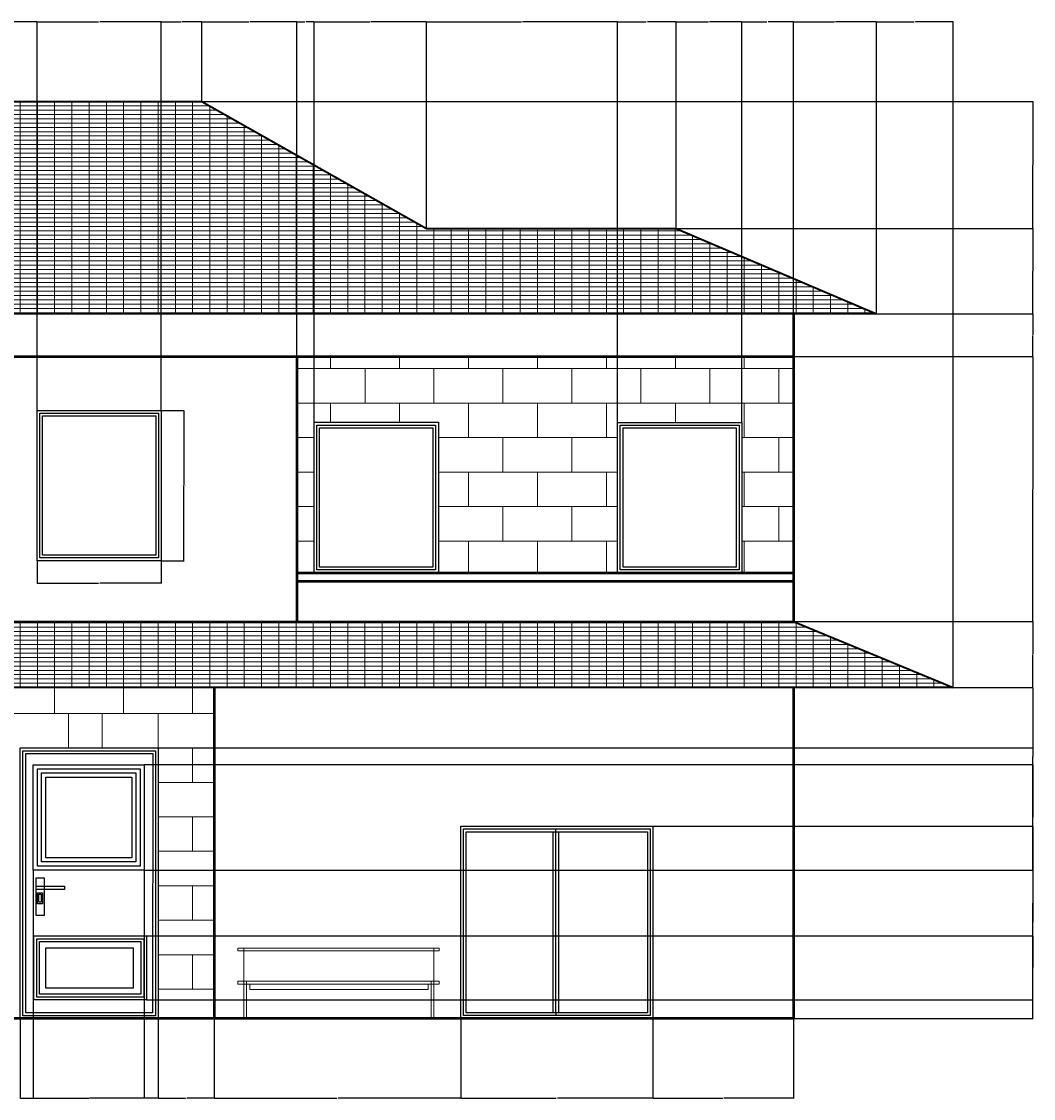
# Model space of a CAD drawing. Units: inches. Extents: x 357 to 1610, y 271 to 1052.
# Tile 2 of 2: x 876 to 1610, y 271 to 1052. Entities that reach past the tile are written whole.
import ezdxf

# ---------------------------------------------------------------- set-up
doc = ezdxf.new("R2010")
doc.units = ezdxf.units.IN
doc.header["$MEASUREMENT"] = 0
for name, color, linetype, lineweight in [('A-ANNO-DIMS', 2, 'Continuous', 18), ('A-DOOR', 40, 'Continuous', 25), ('A-FURN', 40, 'Continuous', 18), ('A-GLAZ', 4, 'Continuous', 25), ('A-ROOF', 7, 'Continuous', 35), ('A-ROOF-PATT', 8, 'Continuous', 13), ('A-WALL', 7, 'Continuous', 50), ('A-WALL-PATT', 8, 'Continuous', 18)]:
    doc.layers.add(name, color=color, linetype=linetype, lineweight=lineweight)
doc.styles.get("Standard").update_dxf_attribs({"font": 'arial.ttf'})
doc.dimstyles.get("Standard").update_dxf_attribs({"dimtxt": 0.18, "dimasz": 0.18, "dimexe": 0.18, "dimexo": 0.0625, "dimgap": 0.09, "dimtad": 0, "dimtih": 1, "dimtoh": 1, "dimdec": 4, "dimzin": 0, "dimdsep": 46, "dimtxsty": 'Standard', "dimcen": 0.09, "dimadec": 0, "dimazin": 0, "dimtfac": 1, "dimtdec": 4, "dimtofl": 0, "dimtmove": 0, "dimatfit": 3, "dimfxl": 1, "dimtolj": 1, "dimtzin": 0, "dimarcsym": 0})

# ---------------------------------------------------------------- blocks, each defined once
blk = doc.blocks.new('WIN-900x1090')
for points in [[(0, 108.96), (90.12, 108.96), (90.12, 0), (0, 0)], [(2, 106.96), (88.12, 106.96), (88.12, 2), (2, 2)], [(4, 104.96), (86.12, 104.96), (86.12, 4), (4, 4)]]:
    blk.add_lwpolyline(points, close=True)
blk = doc.blocks.new('*D2')
at = {"layer": 'A-ANNO-DIMS', "color": 0, "lineweight": -2, "transparency": 16777216}
for p, q in [((977.41, 769.73), (993.87, 769.73)), ((993.69, 769.55), (993.69, 715.44)), ((993.69, 660.95), (993.69, 715.07)), ((977.41, 660.77), (993.87, 660.77))]:
    blk.add_line(p, q, dxfattribs=at)
at = {"layer": 'A-ANNO-DIMS', "color": 0, "transparency": 16777216}
for points in [[(993.66, 769.55), (993.72, 769.55), (993.69, 769.73)], [(993.66, 660.95), (993.72, 660.95), (993.69, 660.77)]]:
    blk.add_solid(points, dxfattribs=at)
at = {"layer": 'Defpoints', "color": 0, "transparency": 16777216}
for p in [(977.34, 769.73), (993.69, 769.73), (977.34, 660.77)]:
    blk.add_point(p, dxfattribs=at)
at = {"layer": 'A-ANNO-DIMS', "color": 0, "transparency": 16777216, "insert": (993.69, 715.25), "char_height": 0.18, "attachment_point": 5}
blk.add_mtext('\\A1;WINDOW 900X1090 109 TYP.', dxfattribs=at)
blk = doc.blocks.new('*D3')
at = {"layer": 'A-ANNO-DIMS', "color": 0, "lineweight": -2, "transparency": 16777216}
for p, q in [((887.22, 660.71), (887.22, 644.25)), ((977.34, 660.71), (977.34, 644.25)), ((887.4, 644.43), (931.75, 644.43)), ((977.16, 644.43), (932.81, 644.43))]:
    blk.add_line(p, q, dxfattribs=at)
at = {"layer": 'A-ANNO-DIMS', "color": 0, "transparency": 16777216}
for points in [[(887.4, 644.46), (887.4, 644.4), (887.22, 644.43)], [(977.16, 644.46), (977.16, 644.4), (977.34, 644.43)]]:
    blk.add_solid(points, dxfattribs=at)
at = {"layer": 'Defpoints', "color": 0, "transparency": 16777216}
for p in [(887.22, 660.77), (977.34, 660.77), (977.34, 644.43)]:
    blk.add_point(p, dxfattribs=at)
at = {"layer": 'A-ANNO-DIMS', "color": 0, "transparency": 16777216, "insert": (932.28, 644.43), "char_height": 0.18, "attachment_point": 5}
blk.add_mtext('\\A1;90 TYP.', dxfattribs=at)
blk = doc.blocks.new('*D10')
at = {"layer": 'A-ANNO-DIMS', "color": 0, "lineweight": -2, "transparency": 16777216}
for p, q in [((835.67, 808.83), (835.67, 1051.75)), ((835.85, 1051.57), (861.05, 1051.57)), ((887.04, 1051.57), (861.84, 1051.57)), ((887.22, 769.8), (887.22, 1051.75))]:
    blk.add_line(p, q, dxfattribs=at)
at = {"layer": 'A-ANNO-DIMS', "color": 0, "transparency": 16777216}
for points in [[(835.85, 1051.6), (835.85, 1051.54), (835.67, 1051.57)], [(887.04, 1051.6), (887.04, 1051.54), (887.22, 1051.57)]]:
    blk.add_solid(points, dxfattribs=at)
at = {"layer": 'Defpoints', "color": 0, "transparency": 16777216}
for p in [(887.22, 1051.57), (835.67, 808.77), (887.22, 769.73)]:
    blk.add_point(p, dxfattribs=at)
at = {"layer": 'A-ANNO-DIMS', "color": 0, "transparency": 16777216, "insert": (861.44, 1051.57), "char_height": 0.18, "attachment_point": 5}
blk.add_mtext('\\A1;51.55', dxfattribs=at)
blk = doc.blocks.new('*D11')
at = {"layer": 'A-ANNO-DIMS', "color": 0, "lineweight": -2, "transparency": 16777216}
for p, q in [((887.22, 769.8), (887.22, 1051.75)), ((887.4, 1051.57), (931.89, 1051.57)), ((977.16, 1051.57), (932.67, 1051.57)), ((977.34, 769.8), (977.34, 1051.75))]:
    blk.add_line(p, q, dxfattribs=at)
at = {"layer": 'A-ANNO-DIMS', "color": 0, "transparency": 16777216}
for points in [[(887.4, 1051.6), (887.4, 1051.54), (887.22, 1051.57)], [(977.16, 1051.6), (977.16, 1051.54), (977.34, 1051.57)]]:
    blk.add_solid(points, dxfattribs=at)
at = {"layer": 'Defpoints', "color": 0, "transparency": 16777216}
for p in [(977.34, 1051.57), (887.22, 769.73), (977.34, 769.73)]:
    blk.add_point(p, dxfattribs=at)
at = {"layer": 'A-ANNO-DIMS', "color": 0, "transparency": 16777216, "insert": (932.28, 1051.57), "char_height": 0.18, "attachment_point": 5}
blk.add_mtext('\\A1;90.12', dxfattribs=at)
blk = doc.blocks.new('*D12')
at = {"layer": 'A-ANNO-DIMS', "color": 0, "lineweight": -2, "transparency": 16777216}
for p, q in [((977.34, 769.8), (977.34, 1051.75)), ((977.52, 1051.57), (991.72, 1051.57)), ((1006.56, 1051.57), (992.37, 1051.57)), ((1006.74, 993.83), (1006.74, 1051.75))]:
    blk.add_line(p, q, dxfattribs=at)
at = {"layer": 'A-ANNO-DIMS', "color": 0, "transparency": 16777216}
for points in [[(977.52, 1051.6), (977.52, 1051.54), (977.34, 1051.57)], [(1006.56, 1051.6), (1006.56, 1051.54), (1006.74, 1051.57)]]:
    blk.add_solid(points, dxfattribs=at)
at = {"layer": 'Defpoints', "color": 0, "transparency": 16777216}
for p in [(1006.74, 1051.57), (1006.74, 993.77), (977.34, 769.73)]:
    blk.add_point(p, dxfattribs=at)
at = {"layer": 'A-ANNO-DIMS', "color": 0, "transparency": 16777216, "insert": (992.04, 1051.57), "char_height": 0.18, "attachment_point": 5}
blk.add_mtext('\\A1;29.4', dxfattribs=at)
blk = doc.blocks.new('*D13')
at = {"layer": 'A-ANNO-DIMS', "color": 0, "lineweight": -2, "transparency": 16777216}
for p, q in [((1006.74, 993.83), (1006.74, 1051.75)), ((1006.92, 1051.57), (1040.81, 1051.57)), ((1075.49, 1051.57), (1041.6, 1051.57)), ((1075.67, 808.83), (1075.67, 1051.75))]:
    blk.add_line(p, q, dxfattribs=at)
at = {"layer": 'A-ANNO-DIMS', "color": 0, "transparency": 16777216}
for points in [[(1006.92, 1051.6), (1006.92, 1051.54), (1006.74, 1051.57)], [(1075.49, 1051.6), (1075.49, 1051.54), (1075.67, 1051.57)]]:
    blk.add_solid(points, dxfattribs=at)
at = {"layer": 'Defpoints', "color": 0, "transparency": 16777216}
for p in [(1075.67, 1051.57), (1006.74, 993.77), (1075.67, 808.77)]:
    blk.add_point(p, dxfattribs=at)
at = {"layer": 'A-ANNO-DIMS', "color": 0, "transparency": 16777216, "insert": (1041.21, 1051.57), "char_height": 0.18, "attachment_point": 5}
blk.add_mtext('\\A1;68.93', dxfattribs=at)
blk = doc.blocks.new('*D14')
at = {"layer": 'A-ANNO-DIMS', "color": 0, "lineweight": -2, "transparency": 16777216}
for p, q in [((1075.67, 808.83), (1075.67, 1051.75)), ((1075.85, 1051.57), (1081.44, 1051.57)), ((1087.93, 1051.57), (1082.35, 1051.57)), ((1088.11, 761.21), (1088.11, 1051.75))]:
    blk.add_line(p, q, dxfattribs=at)
at = {"layer": 'A-ANNO-DIMS', "color": 0, "transparency": 16777216}
for points in [[(1075.85, 1051.6), (1075.85, 1051.54), (1075.67, 1051.57)], [(1087.93, 1051.6), (1087.93, 1051.54), (1088.11, 1051.57)]]:
    blk.add_solid(points, dxfattribs=at)
at = {"layer": 'Defpoints', "color": 0, "transparency": 16777216}
for p in [(1088.11, 1051.57), (1075.67, 808.77), (1088.11, 761.15)]:
    blk.add_point(p, dxfattribs=at)
at = {"layer": 'A-ANNO-DIMS', "color": 0, "transparency": 16777216, "insert": (1081.89, 1051.57), "char_height": 0.18, "attachment_point": 5}
blk.add_mtext('\\A1;12.443', dxfattribs=at)
blk = doc.blocks.new('*D15')
at = {"layer": 'A-ANNO-DIMS', "color": 0, "lineweight": -2, "transparency": 16777216}
for p, q in [((1088.11, 761.21), (1088.11, 1051.75)), ((1088.29, 1051.57), (1128.49, 1051.57)), ((1169.34, 1051.57), (1129.14, 1051.57)), ((1169.52, 901.81), (1169.52, 1051.75))]:
    blk.add_line(p, q, dxfattribs=at)
at = {"layer": 'A-ANNO-DIMS', "color": 0, "transparency": 16777216}
for points in [[(1088.29, 1051.6), (1088.29, 1051.54), (1088.11, 1051.57)], [(1169.34, 1051.6), (1169.34, 1051.54), (1169.52, 1051.57)]]:
    blk.add_solid(points, dxfattribs=at)
at = {"layer": 'Defpoints', "color": 0, "transparency": 16777216}
for p in [(1169.52, 1051.57), (1169.52, 901.75), (1088.11, 761.15)]:
    blk.add_point(p, dxfattribs=at)
at = {"layer": 'A-ANNO-DIMS', "color": 0, "transparency": 16777216, "insert": (1128.82, 1051.57), "char_height": 0.18, "attachment_point": 5}
blk.add_mtext('\\A1;81.4', dxfattribs=at)
blk = doc.blocks.new('*D16')
at = {"layer": 'A-ANNO-DIMS', "color": 0, "lineweight": -2, "transparency": 16777216}
for p, q in [((1169.52, 901.81), (1169.52, 1051.75)), ((1169.7, 1051.57), (1238.43, 1051.57)), ((1307.93, 1051.57), (1239.2, 1051.57)), ((1308.11, 761.12), (1308.11, 1051.75))]:
    blk.add_line(p, q, dxfattribs=at)
at = {"layer": 'A-ANNO-DIMS', "color": 0, "transparency": 16777216}
for points in [[(1169.7, 1051.6), (1169.7, 1051.54), (1169.52, 1051.57)], [(1307.93, 1051.6), (1307.93, 1051.54), (1308.11, 1051.57)]]:
    blk.add_solid(points, dxfattribs=at)
at = {"layer": 'Defpoints', "color": 0, "transparency": 16777216}
for p in [(1308.11, 1051.57), (1169.52, 901.75), (1308.11, 761.06)]:
    blk.add_point(p, dxfattribs=at)
at = {"layer": 'A-ANNO-DIMS', "color": 0, "transparency": 16777216, "insert": (1238.81, 1051.57), "char_height": 0.18, "attachment_point": 5}
blk.add_mtext('\\A1;138.6', dxfattribs=at)
blk = doc.blocks.new('*D17')
at = {"layer": 'A-ANNO-DIMS', "color": 0, "lineweight": -2, "transparency": 16777216}
for p, q in [((1308.11, 761.12), (1308.11, 1051.75)), ((1308.29, 1051.57), (1328.95, 1051.57)), ((1350.4, 1051.57), (1329.74, 1051.57)), ((1350.58, 901.81), (1350.58, 1051.75))]:
    blk.add_line(p, q, dxfattribs=at)
at = {"layer": 'A-ANNO-DIMS', "color": 0, "transparency": 16777216}
for points in [[(1308.29, 1051.6), (1308.29, 1051.54), (1308.11, 1051.57)], [(1350.4, 1051.6), (1350.4, 1051.54), (1350.58, 1051.57)]]:
    blk.add_solid(points, dxfattribs=at)
at = {"layer": 'Defpoints', "color": 0, "transparency": 16777216}
for p in [(1350.58, 1051.57), (1350.58, 901.75), (1308.11, 761.06)]:
    blk.add_point(p, dxfattribs=at)
at = {"layer": 'A-ANNO-DIMS', "color": 0, "transparency": 16777216, "insert": (1329.35, 1051.57), "char_height": 0.18, "attachment_point": 5}
blk.add_mtext('\\A1;42.48', dxfattribs=at)
blk = doc.blocks.new('*D18')
at = {"layer": 'A-ANNO-DIMS', "color": 0, "lineweight": -2, "transparency": 16777216}
for p, q in [((1350.58, 901.81), (1350.58, 1051.75)), ((1350.76, 1051.57), (1374.01, 1051.57)), ((1398.05, 1051.57), (1374.81, 1051.57)), ((1398.23, 761.12), (1398.23, 1051.75))]:
    blk.add_line(p, q, dxfattribs=at)
at = {"layer": 'A-ANNO-DIMS', "color": 0, "transparency": 16777216}
for points in [[(1350.76, 1051.6), (1350.76, 1051.54), (1350.58, 1051.57)], [(1398.05, 1051.6), (1398.05, 1051.54), (1398.23, 1051.57)]]:
    blk.add_solid(points, dxfattribs=at)
at = {"layer": 'Defpoints', "color": 0, "transparency": 16777216}
for p in [(1398.23, 1051.57), (1350.58, 901.75), (1398.23, 761.06)]:
    blk.add_point(p, dxfattribs=at)
at = {"layer": 'A-ANNO-DIMS', "color": 0, "transparency": 16777216, "insert": (1374.41, 1051.57), "char_height": 0.18, "attachment_point": 5}
blk.add_mtext('\\A1;47.65', dxfattribs=at)
blk = doc.blocks.new('*D19')
at = {"layer": 'A-ANNO-DIMS', "color": 0, "lineweight": -2, "transparency": 16777216}
for p, q in [((1398.23, 761.12), (1398.23, 1051.75)), ((1398.41, 1051.57), (1416.45, 1051.57)), ((1435.41, 1051.57), (1417.37, 1051.57)), ((1435.59, 839.95), (1435.59, 1051.75))]:
    blk.add_line(p, q, dxfattribs=at)
at = {"layer": 'A-ANNO-DIMS', "color": 0, "transparency": 16777216}
for points in [[(1398.41, 1051.6), (1398.41, 1051.54), (1398.23, 1051.57)], [(1435.41, 1051.6), (1435.41, 1051.54), (1435.59, 1051.57)]]:
    blk.add_solid(points, dxfattribs=at)
at = {"layer": 'Defpoints', "color": 0, "transparency": 16777216}
for p in [(1435.59, 1051.57), (1435.59, 839.89), (1398.23, 761.06)]:
    blk.add_point(p, dxfattribs=at)
at = {"layer": 'A-ANNO-DIMS', "color": 0, "transparency": 16777216, "insert": (1416.91, 1051.57), "char_height": 0.18, "attachment_point": 5}
blk.add_mtext('\\A1;37.356', dxfattribs=at)
blk = doc.blocks.new('*D20')
at = {"layer": 'A-ANNO-DIMS', "color": 0, "lineweight": -2, "transparency": 16777216}
for p, q in [((1435.59, 839.95), (1435.59, 1051.75)), ((1435.77, 1051.57), (1465.3, 1051.57)), ((1495.63, 1051.57), (1466.09, 1051.57)), ((1495.81, 839.95), (1495.81, 1051.75))]:
    blk.add_line(p, q, dxfattribs=at)
at = {"layer": 'A-ANNO-DIMS', "color": 0, "transparency": 16777216}
for points in [[(1435.77, 1051.6), (1435.77, 1051.54), (1435.59, 1051.57)], [(1495.63, 1051.6), (1495.63, 1051.54), (1495.81, 1051.57)]]:
    blk.add_solid(points, dxfattribs=at)
at = {"layer": 'Defpoints', "color": 0, "transparency": 16777216}
for p in [(1495.81, 1051.57), (1435.59, 839.89), (1495.81, 839.89)]:
    blk.add_point(p, dxfattribs=at)
at = {"layer": 'A-ANNO-DIMS', "color": 0, "transparency": 16777216, "insert": (1465.7, 1051.57), "char_height": 0.18, "attachment_point": 5}
blk.add_mtext('\\A1;60.22', dxfattribs=at)
blk = doc.blocks.new('*D21')
at = {"layer": 'A-ANNO-DIMS', "color": 0, "lineweight": -2, "transparency": 16777216}
for p, q in [((1495.81, 839.95), (1495.81, 1051.75)), ((1495.99, 1051.57), (1523.25, 1051.57)), ((1551.3, 1051.57), (1524.04, 1051.57)), ((1551.48, 568.83), (1551.48, 1051.75))]:
    blk.add_line(p, q, dxfattribs=at)
at = {"layer": 'A-ANNO-DIMS', "color": 0, "transparency": 16777216}
for points in [[(1495.99, 1051.6), (1495.99, 1051.54), (1495.81, 1051.57)], [(1551.3, 1051.6), (1551.3, 1051.54), (1551.48, 1051.57)]]:
    blk.add_solid(points, dxfattribs=at)
at = {"layer": 'Defpoints', "color": 0, "transparency": 16777216}
for p in [(1551.48, 1051.57), (1495.81, 839.89), (1551.48, 568.77)]:
    blk.add_point(p, dxfattribs=at)
at = {"layer": 'A-ANNO-DIMS', "color": 0, "transparency": 16777216, "insert": (1523.64, 1051.57), "char_height": 0.18, "attachment_point": 5}
blk.add_mtext('\\A1;55.67', dxfattribs=at)
blk = doc.blocks.new('*D27')
at = {"layer": 'A-ANNO-DIMS', "color": 0, "lineweight": -2, "transparency": 16777216}
for p, q in [((875, 328.7), (875, 270.79)), ((975, 328.7), (975, 270.79)), ((875.18, 270.97), (924.72, 270.97)), ((974.82, 270.97), (925.28, 270.97))]:
    blk.add_line(p, q, dxfattribs=at)
at = {"layer": 'A-ANNO-DIMS', "color": 0, "transparency": 16777216}
for points in [[(875.18, 271), (875.18, 270.94), (875, 270.97)], [(974.82, 271), (974.82, 270.94), (975, 270.97)]]:
    blk.add_solid(points, dxfattribs=at)
at = {"layer": 'Defpoints', "color": 0, "transparency": 16777216}
for p in [(875, 328.77), (975, 328.77), (975, 270.97)]:
    blk.add_point(p, dxfattribs=at)
at = {"layer": 'A-ANNO-DIMS', "color": 0, "transparency": 16777216, "insert": (925, 270.97), "char_height": 0.18, "attachment_point": 5}
blk.add_mtext('\\A1;100', dxfattribs=at)
blk = doc.blocks.new('*D28')
at = {"layer": 'A-ANNO-DIMS', "color": 0, "lineweight": -2, "transparency": 16777216}
for p, q in [((975, 328.7), (975, 270.79)), ((1015.67, 328.7), (1015.67, 270.79)), ((975.18, 270.97), (994.94, 270.97)), ((1015.49, 270.97), (995.73, 270.97))]:
    blk.add_line(p, q, dxfattribs=at)
at = {"layer": 'A-ANNO-DIMS', "color": 0, "transparency": 16777216}
for points in [[(975.18, 271), (975.18, 270.94), (975, 270.97)], [(1015.49, 271), (1015.49, 270.94), (1015.67, 270.97)]]:
    blk.add_solid(points, dxfattribs=at)
at = {"layer": 'Defpoints', "color": 0, "transparency": 16777216}
for p in [(975, 328.77), (1015.67, 328.77), (1015.67, 270.97)]:
    blk.add_point(p, dxfattribs=at)
at = {"layer": 'A-ANNO-DIMS', "color": 0, "transparency": 16777216, "insert": (995.33, 270.97), "char_height": 0.18, "attachment_point": 5}
blk.add_mtext('\\A1;40.67', dxfattribs=at)
blk = doc.blocks.new('*D29')
at = {"layer": 'A-ANNO-DIMS', "color": 0, "lineweight": -2, "transparency": 16777216}
for p, q in [((1015.67, 328.7), (1015.67, 270.79)), ((1194.43, 328.82), (1194.43, 270.79)), ((1015.85, 270.97), (1104.6, 270.97)), ((1194.25, 270.97), (1105.51, 270.97))]:
    blk.add_line(p, q, dxfattribs=at)
at = {"layer": 'A-ANNO-DIMS', "color": 0, "transparency": 16777216}
for points in [[(1015.85, 271), (1015.85, 270.94), (1015.67, 270.97)], [(1194.25, 271), (1194.25, 270.94), (1194.43, 270.97)]]:
    blk.add_solid(points, dxfattribs=at)
at = {"layer": 'Defpoints', "color": 0, "transparency": 16777216}
for p in [(1015.67, 328.77), (1194.43, 328.88), (1194.43, 270.97)]:
    blk.add_point(p, dxfattribs=at)
at = {"layer": 'A-ANNO-DIMS', "color": 0, "transparency": 16777216, "insert": (1105.05, 270.97), "char_height": 0.18, "attachment_point": 5}
blk.add_mtext('\\A1;178.76', dxfattribs=at)
blk = doc.blocks.new('*D30')
at = {"layer": 'A-ANNO-DIMS', "color": 0, "lineweight": -2, "transparency": 16777216}
for p, q in [((1194.43, 328.82), (1194.43, 270.79)), ((1333.76, 328.82), (1333.76, 270.79)), ((1194.61, 270.97), (1263.64, 270.97)), ((1333.58, 270.97), (1264.55, 270.97))]:
    blk.add_line(p, q, dxfattribs=at)
at = {"layer": 'A-ANNO-DIMS', "color": 0, "transparency": 16777216}
for points in [[(1194.61, 271), (1194.61, 270.94), (1194.43, 270.97)], [(1333.58, 271), (1333.58, 270.94), (1333.76, 270.97)]]:
    blk.add_solid(points, dxfattribs=at)
at = {"layer": 'Defpoints', "color": 0, "transparency": 16777216}
for p in [(1194.43, 328.88), (1333.76, 328.88), (1333.76, 270.97)]:
    blk.add_point(p, dxfattribs=at)
at = {"layer": 'A-ANNO-DIMS', "color": 0, "transparency": 16777216, "insert": (1264.1, 270.97), "char_height": 0.18, "attachment_point": 5}
blk.add_mtext('\\A1;139.33', dxfattribs=at)
blk = doc.blocks.new('*D31')
at = {"layer": 'A-ANNO-DIMS', "color": 0, "lineweight": -2, "transparency": 16777216}
for p, q in [((1333.76, 328.82), (1333.76, 270.79)), ((1435.67, 328.7), (1435.67, 270.79)), ((1333.94, 270.97), (1384.33, 270.97)), ((1435.49, 270.97), (1385.1, 270.97))]:
    blk.add_line(p, q, dxfattribs=at)
at = {"layer": 'A-ANNO-DIMS', "color": 0, "transparency": 16777216}
for points in [[(1333.94, 271), (1333.94, 270.94), (1333.76, 270.97)], [(1435.49, 271), (1435.49, 270.94), (1435.67, 270.97)]]:
    blk.add_solid(points, dxfattribs=at)
at = {"layer": 'Defpoints', "color": 0, "transparency": 16777216}
for p in [(1333.76, 328.88), (1435.67, 328.77), (1435.67, 270.97)]:
    blk.add_point(p, dxfattribs=at)
at = {"layer": 'A-ANNO-DIMS', "color": 0, "transparency": 16777216, "insert": (1384.71, 270.97), "char_height": 0.18, "attachment_point": 5}
blk.add_mtext('\\A1;101.9', dxfattribs=at)
blk = doc.blocks.new('*D40')
at = {"layer": 'A-ANNO-DIMS', "color": 0, "lineweight": -2, "transparency": 16777216}
for p, q in [((1194.5, 468.2), (1609.46, 468.2)), ((1609.28, 468.02), (1609.28, 398.67)), ((1609.28, 328.95), (1609.28, 398.3)), ((1435.73, 328.77), (1609.46, 328.77))]:
    blk.add_line(p, q, dxfattribs=at)
at = {"layer": 'A-ANNO-DIMS', "color": 0, "transparency": 16777216}
for points in [[(1609.25, 468.02), (1609.31, 468.02), (1609.28, 468.2)], [(1609.25, 328.95), (1609.31, 328.95), (1609.28, 328.77)]]:
    blk.add_solid(points, dxfattribs=at)
at = {"layer": 'Defpoints', "color": 0, "transparency": 16777216}
for p in [(1194.43, 468.2), (1609.28, 468.2), (1435.67, 328.77)]:
    blk.add_point(p, dxfattribs=at)
at = {"layer": 'A-ANNO-DIMS', "color": 0, "transparency": 16777216, "insert": (1609.28, 398.49), "char_height": 0.18, "attachment_point": 5}
blk.add_mtext('\\A1;139.44', dxfattribs=at)
blk = doc.blocks.new('*D41')
at = {"layer": 'A-ANNO-DIMS', "color": 0, "lineweight": -2, "transparency": 16777216}
for p, q in [((1551.54, 568.77), (1609.46, 568.77)), ((1609.28, 568.59), (1609.28, 518.67)), ((1609.28, 468.38), (1609.28, 518.3)), ((1194.5, 468.2), (1609.46, 468.2))]:
    blk.add_line(p, q, dxfattribs=at)
at = {"layer": 'A-ANNO-DIMS', "color": 0, "transparency": 16777216}
for points in [[(1609.25, 568.59), (1609.31, 568.59), (1609.28, 568.77)], [(1609.25, 468.38), (1609.31, 468.38), (1609.28, 468.2)]]:
    blk.add_solid(points, dxfattribs=at)
at = {"layer": 'Defpoints', "color": 0, "transparency": 16777216}
for p in [(1551.48, 568.77), (1609.28, 568.77), (1194.43, 468.2)]:
    blk.add_point(p, dxfattribs=at)
at = {"layer": 'A-ANNO-DIMS', "color": 0, "transparency": 16777216, "insert": (1609.28, 518.49), "char_height": 0.18, "attachment_point": 5}
blk.add_mtext('\\A1;100.56', dxfattribs=at)
blk = doc.blocks.new('*D42')
at = {"layer": 'A-ANNO-DIMS', "color": 0, "lineweight": -2, "transparency": 16777216}
for p, q in [((1435.73, 616.77), (1609.46, 616.77)), ((1609.28, 616.59), (1609.28, 592.95)), ((1609.28, 568.95), (1609.28, 592.59)), ((1551.54, 568.77), (1609.46, 568.77))]:
    blk.add_line(p, q, dxfattribs=at)
at = {"layer": 'A-ANNO-DIMS', "color": 0, "transparency": 16777216}
for points in [[(1609.25, 616.59), (1609.31, 616.59), (1609.28, 616.77)], [(1609.25, 568.95), (1609.31, 568.95), (1609.28, 568.77)]]:
    blk.add_solid(points, dxfattribs=at)
at = {"layer": 'Defpoints', "color": 0, "transparency": 16777216}
for p in [(1435.67, 616.77), (1609.28, 616.77), (1551.48, 568.77)]:
    blk.add_point(p, dxfattribs=at)
at = {"layer": 'A-ANNO-DIMS', "color": 0, "transparency": 16777216, "insert": (1609.28, 592.77), "char_height": 0.18, "attachment_point": 5}
blk.add_mtext('\\A1;48', dxfattribs=at)
blk = doc.blocks.new('*D43')
at = {"layer": 'A-ANNO-DIMS', "color": 0, "lineweight": -2, "transparency": 16777216}
for p, q in [((1075.73, 808.77), (1609.46, 808.77)), ((1609.28, 808.59), (1609.28, 712.95)), ((1609.28, 616.95), (1609.28, 712.59)), ((1435.73, 616.77), (1609.46, 616.77))]:
    blk.add_line(p, q, dxfattribs=at)
at = {"layer": 'A-ANNO-DIMS', "color": 0, "transparency": 16777216}
for points in [[(1609.25, 808.59), (1609.31, 808.59), (1609.28, 808.77)], [(1609.25, 616.95), (1609.31, 616.95), (1609.28, 616.77)]]:
    blk.add_solid(points, dxfattribs=at)
at = {"layer": 'Defpoints', "color": 0, "transparency": 16777216}
for p in [(1075.67, 808.77), (1609.28, 808.77), (1435.67, 616.77)]:
    blk.add_point(p, dxfattribs=at)
at = {"layer": 'A-ANNO-DIMS', "color": 0, "transparency": 16777216, "insert": (1609.28, 712.77), "char_height": 0.18, "attachment_point": 5}
blk.add_mtext('\\A1;192', dxfattribs=at)
blk = doc.blocks.new('*D44')
at = {"layer": 'A-ANNO-DIMS', "color": 0, "lineweight": -2, "transparency": 16777216}
for p, q in [((1495.87, 839.89), (1609.46, 839.89)), ((1609.28, 839.71), (1609.28, 824.51)), ((1609.28, 808.95), (1609.28, 824.15)), ((1075.73, 808.77), (1609.46, 808.77))]:
    blk.add_line(p, q, dxfattribs=at)
at = {"layer": 'A-ANNO-DIMS', "color": 0, "transparency": 16777216}
for points in [[(1609.25, 839.71), (1609.31, 839.71), (1609.28, 839.89)], [(1609.25, 808.95), (1609.31, 808.95), (1609.28, 808.77)]]:
    blk.add_solid(points, dxfattribs=at)
at = {"layer": 'Defpoints', "color": 0, "transparency": 16777216}
for p in [(1495.81, 839.89), (1609.28, 839.89), (1075.67, 808.77)]:
    blk.add_point(p, dxfattribs=at)
at = {"layer": 'A-ANNO-DIMS', "color": 0, "transparency": 16777216, "insert": (1609.28, 824.33), "char_height": 0.18, "attachment_point": 5}
blk.add_mtext('\\A1;31.12', dxfattribs=at)
blk = doc.blocks.new('*D45')
at = {"layer": 'A-ANNO-DIMS', "color": 0, "lineweight": -2, "transparency": 16777216}
for p, q in [((1350.65, 901.75), (1609.46, 901.75)), ((1609.28, 901.57), (1609.28, 871)), ((1609.28, 840.07), (1609.28, 870.64)), ((1495.87, 839.89), (1609.46, 839.89))]:
    blk.add_line(p, q, dxfattribs=at)
at = {"layer": 'A-ANNO-DIMS', "color": 0, "transparency": 16777216}
for points in [[(1609.25, 901.57), (1609.31, 901.57), (1609.28, 901.75)], [(1609.25, 840.07), (1609.31, 840.07), (1609.28, 839.89)]]:
    blk.add_solid(points, dxfattribs=at)
at = {"layer": 'Defpoints', "color": 0, "transparency": 16777216}
for p in [(1350.58, 901.75), (1609.28, 901.75), (1495.81, 839.89)]:
    blk.add_point(p, dxfattribs=at)
at = {"layer": 'A-ANNO-DIMS', "color": 0, "transparency": 16777216, "insert": (1609.28, 870.82), "char_height": 0.18, "attachment_point": 5}
blk.add_mtext('\\A1;61.86', dxfattribs=at)
blk = doc.blocks.new('*D46')
at = {"layer": 'A-ANNO-DIMS', "color": 0, "lineweight": -2, "transparency": 16777216}
for p, q in [((1006.8, 993.77), (1609.46, 993.77)), ((1609.28, 993.59), (1609.28, 947.94)), ((1609.28, 901.93), (1609.28, 947.58)), ((1350.65, 901.75), (1609.46, 901.75))]:
    blk.add_line(p, q, dxfattribs=at)
at = {"layer": 'A-ANNO-DIMS', "color": 0, "transparency": 16777216}
for points in [[(1609.25, 993.59), (1609.31, 993.59), (1609.28, 993.77)], [(1609.25, 901.93), (1609.31, 901.93), (1609.28, 901.75)]]:
    blk.add_solid(points, dxfattribs=at)
at = {"layer": 'Defpoints', "color": 0, "transparency": 16777216}
for p in [(1006.74, 993.77), (1609.28, 993.77), (1350.58, 901.75)]:
    blk.add_point(p, dxfattribs=at)
at = {"layer": 'A-ANNO-DIMS', "color": 0, "transparency": 16777216, "insert": (1609.28, 947.76), "char_height": 0.18, "attachment_point": 5}
blk.add_mtext('\\A1;92.02', dxfattribs=at)
blk = doc.blocks.new('*D47')
at = {"layer": 'A-ANNO-DIMS', "color": 0, "lineweight": -2, "transparency": 16777216}
for p, q in [((966.64, 388.65), (1609.46, 388.65)), ((1609.28, 388.47), (1609.28, 365.69)), ((1609.28, 342.54), (1609.28, 365.32)), ((966.64, 342.36), (1609.46, 342.36))]:
    blk.add_line(p, q, dxfattribs=at)
at = {"layer": 'A-ANNO-DIMS', "color": 0, "transparency": 16777216}
for points in [[(1609.25, 388.47), (1609.31, 388.47), (1609.28, 388.65)], [(1609.25, 342.54), (1609.31, 342.54), (1609.28, 342.36)]]:
    blk.add_solid(points, dxfattribs=at)
at = {"layer": 'Defpoints', "color": 0, "transparency": 16777216}
for p in [(966.57, 388.65), (1609.28, 388.65), (966.57, 342.36)]:
    blk.add_point(p, dxfattribs=at)
at = {"layer": 'A-ANNO-DIMS', "color": 0, "transparency": 16777216, "insert": (1609.28, 365.51), "char_height": 0.18, "attachment_point": 5}
blk.add_mtext('\\A1;46.3', dxfattribs=at)
blk = doc.blocks.new('*D48')
at = {"layer": 'A-ANNO-DIMS', "color": 0, "lineweight": -2, "transparency": 16777216}
for p, q in [((965.04, 436.35), (1609.46, 436.35)), ((1609.28, 436.17), (1609.28, 412.68)), ((1609.28, 388.83), (1609.28, 412.32)), ((966.64, 388.65), (1609.46, 388.65))]:
    blk.add_line(p, q, dxfattribs=at)
at = {"layer": 'A-ANNO-DIMS', "color": 0, "transparency": 16777216}
for points in [[(1609.25, 436.17), (1609.31, 436.17), (1609.28, 436.35)], [(1609.25, 388.83), (1609.31, 388.83), (1609.28, 388.65)]]:
    blk.add_solid(points, dxfattribs=at)
at = {"layer": 'Defpoints', "color": 0, "transparency": 16777216}
for p in [(964.98, 436.35), (1609.28, 436.35), (966.57, 388.65)]:
    blk.add_point(p, dxfattribs=at)
at = {"layer": 'A-ANNO-DIMS', "color": 0, "transparency": 16777216, "insert": (1609.28, 412.5), "char_height": 0.18, "attachment_point": 5}
blk.add_mtext('\\A1;47.7', dxfattribs=at)
blk = doc.blocks.new('*D49')
at = {"layer": 'A-ANNO-DIMS', "color": 0, "lineweight": -2, "transparency": 16777216}
for p, q in [((965.04, 512.85), (1609.46, 512.85)), ((1609.28, 512.67), (1609.28, 474.78)), ((1609.28, 436.53), (1609.28, 474.42)), ((965.04, 436.35), (1609.46, 436.35))]:
    blk.add_line(p, q, dxfattribs=at)
at = {"layer": 'A-ANNO-DIMS', "color": 0, "transparency": 16777216}
for points in [[(1609.25, 512.67), (1609.31, 512.67), (1609.28, 512.85)], [(1609.25, 436.53), (1609.31, 436.53), (1609.28, 436.35)]]:
    blk.add_solid(points, dxfattribs=at)
at = {"layer": 'Defpoints', "color": 0, "transparency": 16777216}
for p in [(964.98, 512.85), (1609.28, 512.85), (964.98, 436.35)]:
    blk.add_point(p, dxfattribs=at)
at = {"layer": 'A-ANNO-DIMS', "color": 0, "transparency": 16777216, "insert": (1609.28, 474.6), "char_height": 0.18, "attachment_point": 5}
blk.add_mtext('\\A1;76.5', dxfattribs=at)
blk = doc.blocks.new('*D50')
at = {"layer": 'A-ANNO-DIMS', "color": 0, "lineweight": -2, "transparency": 16777216}
for p, q in [((975.06, 525), (1609.46, 525)), ((1609.28, 524.82), (1609.28, 519.1)), ((1609.28, 513.03), (1609.28, 518.74)), ((965.04, 512.85), (1609.46, 512.85))]:
    blk.add_line(p, q, dxfattribs=at)
at = {"layer": 'A-ANNO-DIMS', "color": 0, "transparency": 16777216}
for points in [[(1609.25, 524.82), (1609.31, 524.82), (1609.28, 525)], [(1609.25, 513.03), (1609.31, 513.03), (1609.28, 512.85)]]:
    blk.add_solid(points, dxfattribs=at)
at = {"layer": 'Defpoints', "color": 0, "transparency": 16777216}
for p in [(975, 525), (1609.28, 525), (964.98, 512.85)]:
    blk.add_point(p, dxfattribs=at)
at = {"layer": 'A-ANNO-DIMS', "color": 0, "transparency": 16777216, "insert": (1609.28, 518.92), "char_height": 0.18, "attachment_point": 5}
blk.add_mtext('\\A1;12.154', dxfattribs=at)
blk = doc.blocks.new('*D51')
at = {"layer": 'A-ANNO-DIMS', "color": 0, "lineweight": -2, "transparency": 16777216}
for p, q in [((884.54, 436.29), (884.54, 270.79)), ((964.98, 436.29), (964.98, 270.79)), ((884.72, 270.97), (924.37, 270.97)), ((964.8, 270.97), (925.15, 270.97))]:
    blk.add_line(p, q, dxfattribs=at)
at = {"layer": 'A-ANNO-DIMS', "color": 0, "transparency": 16777216}
for points in [[(884.72, 271), (884.72, 270.94), (884.54, 270.97)], [(964.8, 271), (964.8, 270.94), (964.98, 270.97)]]:
    blk.add_solid(points, dxfattribs=at)
at = {"layer": 'Defpoints', "color": 0, "transparency": 16777216}
for p in [(884.54, 436.35), (964.98, 436.35), (964.98, 270.97)]:
    blk.add_point(p, dxfattribs=at)
at = {"layer": 'A-ANNO-DIMS', "color": 0, "transparency": 16777216, "insert": (924.76, 270.97), "char_height": 0.18, "attachment_point": 5}
blk.add_mtext('\\A1;80.44', dxfattribs=at)

msp = doc.modelspace()

# ---------------------------------------------------------------- hatches: boundary and pattern name
at = {"layer": 'A-ROOF-PATT'}
h = msp.add_hatch(dxfattribs=at)
h.set_pattern_fill('GRATE', color=256, scale=100)
h.paths.add_polyline_path([(1006.7419, 993.7706), (702.2918, 993.7706), (415.4488, 839.8897), (475.6698, 839.8897), (1435.5868, 839.8897), (1495.8077, 839.8897), (1350.5849, 901.7507), (1169.5186, 901.7507)])
h = msp.add_hatch(dxfattribs=at)
h.set_pattern_fill('GRATE', color=256, scale=100)
h.paths.add_polyline_path([(1435.6698, 616.7674), (579.8425, 616.7674), (475.6698, 568.7674), (1435.6698, 568.7674), (1551.4751, 568.7674)])
at = {"layer": 'A-WALL-PATT'}
h = msp.add_hatch(dxfattribs=at)
h.set_pattern_fill('BRICK', color=256, scale=100)
h.paths.add_polyline_path([(835.6698, 652.0149), (835.6698, 808.7674), (475.6698, 808.7674), (475.6698, 652.0149), (547.031, 652.0149), (547.031, 760.9583), (637.1546, 760.9583), (637.1546, 652.0149)])
h.paths.add_polyline_path([(699.7613, 761.2521), (789.8849, 761.2521), (789.8849, 652.2919), (699.7613, 652.2919)], flags=16)
h.paths.add_polyline_path([(701.7613, 759.2521), (787.8849, 759.2521), (787.8849, 654.2919), (701.7613, 654.2919)], flags=0)
h.paths.add_polyline_path([(703.7613, 757.2521), (785.8849, 757.2521), (785.8849, 656.2919), (703.7613, 656.2919)], flags=0)
h.paths.add_polyline_path([(1308.107, 761.0593), (1398.2306, 761.0593), (1398.2306, 652.0149), (1435.6698, 652.0149), (1435.6698, 808.7674), (1075.6698, 808.7674), (1075.6698, 652.0149), (1088.1132, 652.0149), (1088.1132, 761.152), (1178.2368, 761.152), (1178.2368, 652.0149), (1308.107, 652.0149)])

# ---------------------------------------------------------------- linework, layer by layer
at = {"layer": 'A-DOOR'}
for p, q in [((1194.4336, 468.2044), (1333.7597, 468.2044)), ((1194.4336, 328.8783), (1194.4336, 468.2044)), ((1196.4336, 466.2044), (1331.7597, 466.2044)), ((1196.4336, 330.8783), (1196.4336, 466.2044)), ((1198.4336, 464.2044), (1329.7597, 464.2044)), ((1198.4336, 332.8783), (1198.4336, 464.2044)), ((1261.4336, 332.8783), (1261.4336, 464.2044)), ((1263.4336, 463.2743), (1263.4336, 466.2044)), ((1263.4336, 332.8783), (1263.4336, 464.2044)), ((1265.4336, 332.8783), (1265.4336, 464.2044)), ((1329.7597, 464.2044), (1329.7597, 332.8783)), ((1331.7597, 466.2044), (1331.7597, 330.8783)), ((1333.7597, 468.2044), (1333.7597, 328.8783)), ((907.1083, 424.8564), (907.1083, 422.2369)), ((1333.7597, 328.8783), (1194.4336, 328.8783)), ((1331.7597, 330.8783), (1196.4336, 330.8783)), ((1329.7597, 332.8783), (1198.4336, 332.8783)), ((1263.4336, 332.8783), (1263.4336, 330.8783))]:
    msp.add_line(p, q, dxfattribs=at)
for points in [[(975, 525), (975.0913, 525), (975, 328.7674), (875, 328.7674), (875, 525)], [(973.0903, 523), (973.0009, 330.7674), (877, 330.7674), (877, 523)], [(971.0894, 521), (971.0019, 332.7674), (879, 332.7674), (879, 521)], [(884.5365, 512.8457), (964.9806, 512.8457), (964.9806, 436.3532), (884.5365, 436.3532)], [(887.5365, 509.8457), (961.9806, 509.8457), (961.9806, 439.3532), (887.5365, 439.3532)], [(890.5365, 506.8457), (958.9806, 506.8457), (958.9806, 442.3532), (890.5365, 442.3532)], [(893.5365, 503.8457), (955.9806, 503.8457), (955.9806, 445.3532), (893.5365, 445.3532)], [(886.5299, 430.794), (892.2976, 430.794), (892.2976, 403.5508), (886.5299, 403.5508)], [(887.496, 419.9028), (891.1527, 419.9028), (891.1527, 412.04), (887.496, 412.04)], [(888.496, 418.9028), (890.1527, 418.9028), (890.1527, 413.04), (888.496, 413.04)], [(884.9669, 388.6534), (966.5742, 388.6534), (966.5742, 342.3568), (884.9669, 342.3568)], [(886.9669, 386.6534), (964.5742, 386.6534), (964.5742, 344.3568), (886.9669, 344.3568)], [(888.9669, 384.6534), (962.5742, 384.6534), (962.5742, 346.3568), (888.9669, 346.3568)], [(893.6343, 380.0645), (956.9771, 380.0645), (956.9771, 350.76), (893.6343, 350.76)]]:
    msp.add_lwpolyline(points, close=True, dxfattribs=at)
for points in [[(886.5299, 424.8564), (907.1083, 424.8564)], [(907.1083, 422.2369), (886.5299, 422.2369)]]:
    msp.add_lwpolyline(points, dxfattribs=at)
at = {"layer": 'A-FURN'}
for p, q in [((1039.0994, 328.7984), (1039.0994, 355.7914)), ((1172.8934, 355.7914), (1172.8934, 328.7984))]:
    msp.add_line(p, q, dxfattribs=at)
for points in [[(1037.0994, 379.7914), (1174.8934, 379.7914), (1174.8934, 328.7984), (1037.0994, 328.7984), (1037.0994, 379.7914), (1032.8195, 379.7914), (1032.8195, 377.7914), (1174.8934, 377.7914), (1178.8699, 377.7914), (1178.8699, 379.7699), (1174.8934, 379.7914)], [(1041.4972, 353.7914), (1041.4972, 349.7914), (1170.9022, 349.7914), (1170.9022, 353.7914)]]:
    msp.add_lwpolyline(points, dxfattribs=at)
msp.add_lwpolyline([(1178.8699, 353.7914), (1178.8699, 355.7914), (1174.8934, 355.7914), (1037.0994, 355.7914), (1032.8195, 355.7914), (1032.8195, 353.7784), (1037.0994, 353.7914), (1174.8934, 353.7914)], close=True, dxfattribs=at)
at = {"layer": 'A-ROOF'}
for points in [[(1435.5868, 839.8897), (475.6698, 839.8897), (415.4488, 839.8897), (702.2918, 993.7706), (1006.7419, 993.7706), (1169.5186, 901.7507), (1350.5849, 901.7507), (1495.8077, 839.8897)], [(1435.6698, 568.7674), (475.6698, 568.7674), (579.8425, 616.7674), (1435.6698, 616.7674), (1551.4751, 568.7674)]]:
    msp.add_lwpolyline(points, close=True, dxfattribs=at)
at = {"layer": 'A-WALL'}
for p, q in [((1435.5868, 839.8897), (1435.5868, 808.7674)), ((475.6698, 808.7674), (1435.6698, 808.7674)), ((1075.6698, 808.7674), (1075.6698, 616.7674)), ((1435.6698, 808.7674), (1435.6698, 616.7674)), ((1075.6698, 652.0149), (1435.6698, 652.0149)), ((1075.6698, 646.0149), (1435.6698, 646.0149)), ((1015.6698, 568.7674), (1015.6698, 328.7674)), ((1435.6698, 568.7674), (1435.6698, 328.7674)), ((1435.6698, 328.7674), (475.6698, 328.7674))]:
    msp.add_line(p, q, dxfattribs=at)
at = {"layer": 'A-WALL-PATT'}
for p, q in [((900, 550), (900, 568.7674)), ((950, 550), (950, 568.7674)), ((1000, 550), (1000, 568.7674)), ((715.6698, 550), (1015.6698, 550)), ((909.955, 550), (909.955, 525)), ((934.4337, 550), (934.4337, 525)), ((975, 525), (975, 550)), ((975, 525), (1015.6698, 525)), ((1000, 500), (1000, 525)), ((975, 475), (975, 500)), ((975, 500), (1015.6698, 500)), ((975, 475), (1015.6698, 475)), ((1000, 450), (1000, 475)), ((975, 425), (975, 450)), ((975, 450), (1015.6698, 450)), ((975, 425), (1015.6698, 425)), ((1000, 400), (1000, 425)), ((975, 375), (975, 400)), ((975, 400), (1015.6698, 400)), ((975, 375), (1015.6698, 375)), ((1000, 350), (1000, 375)), ((975, 328.7674), (975, 350)), ((975, 350), (1015.6698, 350))]:
    msp.add_line(p, q, dxfattribs=at)

# ---------------------------------------------------------------- block references
at = {"layer": 'A-GLAZ'}
for p in [(887.219, 660.774), (1088.1132, 652.1915), (1308.107, 652.0988)]:
    msp.add_blockref('WIN-900x1090', p, dxfattribs=at)

# ---------------------------------------------------------------- dimensions: what is measured, and where the dimension line sits
at = {"layer": 'A-ANNO-DIMS'}
for base, p1, p2, override, picture, middle in [((887.2189, 1051.5706), (835.6698, 808.7674), (887.2189, 769.7345), {"dimdec": 2, "dimlfac": 1, "dimrnd": 0, "dimzin": 0, "dimdsep": 46, "dimlunit": 2}, '*D10', (861.4444, 1051.5706)), ((977.3425, 1051.5706), (887.2189, 769.7345), (977.3425, 769.7345), {"dimdec": 2, "dimlfac": 1, "dimrnd": 0, "dimzin": 0, "dimdsep": 46, "dimlunit": 2}, '*D11', (932.2807, 1051.5706)), ((1006.7419, 1051.5706), (977.3425, 769.7345), (1006.7419, 993.7706), {"dimdec": 1, "dimlfac": 1, "dimrnd": 0, "dimzin": 0, "dimdsep": 46, "dimlunit": 2}, '*D12', (992.0422, 1051.5706)), ((1075.6698, 1051.5706), (1006.7419, 993.7706), (1075.6698, 808.7674), {"dimdec": 2, "dimlfac": 1, "dimrnd": 0, "dimzin": 0, "dimdsep": 46, "dimlunit": 2}, '*D13', (1041.2058, 1051.5706)), ((1088.1132, 1051.5706), (1075.6698, 808.7674), (1088.1132, 761.152), {"dimdec": 3, "dimlfac": 1, "dimrnd": 0, "dimzin": 0, "dimdsep": 46, "dimlunit": 2}, '*D14', (1081.8915, 1051.5706)), ((1169.5186, 1051.5706), (1088.1132, 761.152), (1169.5186, 901.7507), {"dimdec": 1, "dimlfac": 1, "dimrnd": 0, "dimzin": 0, "dimdsep": 46, "dimlunit": 2}, '*D15', (1128.8159, 1051.5706)), ((1308.107, 1051.5706), (1169.5186, 901.7507), (1308.107, 761.0593), {"dimdec": 1, "dimlfac": 1, "dimrnd": 0, "dimzin": 0, "dimdsep": 46, "dimlunit": 2}, '*D16', (1238.8128, 1051.5706)), ((1350.5849, 1051.5706), (1308.107, 761.0593), (1350.5849, 901.7507), {"dimdec": 2, "dimlfac": 1, "dimrnd": 0, "dimzin": 0, "dimdsep": 46, "dimlunit": 2}, '*D17', (1329.346, 1051.5706)), ((1398.2306, 1051.5706), (1350.5849, 901.7507), (1398.2306, 761.0593), {"dimdec": 2, "dimlfac": 1, "dimrnd": 0, "dimzin": 0, "dimdsep": 46, "dimlunit": 2}, '*D18', (1374.4078, 1051.5706)), ((1435.5868, 1051.5706), (1398.2306, 761.0593), (1435.5868, 839.8897), {"dimdec": 3, "dimlfac": 1, "dimrnd": 0, "dimzin": 0, "dimdsep": 46, "dimlunit": 2}, '*D19', (1416.9087, 1051.5706)), ((1495.8077, 1051.5706), (1435.5868, 839.8897), (1495.8077, 839.8897), {"dimdec": 2, "dimlfac": 1, "dimrnd": 0, "dimzin": 0, "dimdsep": 46, "dimlunit": 2}, '*D20', (1465.6973, 1051.5706)), ((1551.4751, 1051.5706), (1495.8077, 839.8897), (1551.4751, 568.7674), {"dimdec": 2, "dimlfac": 1, "dimrnd": 0, "dimzin": 0, "dimdsep": 46, "dimlunit": 2}, '*D21', (1523.6414, 1051.5706)), ((964.9806, 270.9674), (884.5365, 436.3532), (964.9806, 436.3532), {"dimdec": 2, "dimlfac": 1, "dimrnd": 0, "dimzin": 0, "dimdsep": 46, "dimlunit": 2}, '*D51', (924.7586, 270.9674)), ((975, 270.9674), (875, 328.7674), (975, 328.7674), {"dimdec": 0, "dimlfac": 1, "dimrnd": 0, "dimzin": 0, "dimdsep": 46, "dimlunit": 2}, '*D27', (925, 270.9674)), ((1015.6698, 270.9674), (975, 328.7674), (1015.6698, 328.7674), {"dimdec": 2, "dimlfac": 1, "dimrnd": 0, "dimzin": 0, "dimdsep": 46, "dimlunit": 2}, '*D28', (995.3349, 270.9674)), ((1194.4336, 270.9674), (1015.6698, 328.7674), (1194.4336, 328.8783), {"dimdec": 2, "dimlfac": 1, "dimrnd": 0, "dimzin": 0, "dimdsep": 46, "dimlunit": 2}, '*D29', (1105.0517, 270.9674)), ((1333.7597, 270.9674), (1194.4336, 328.8783), (1333.7597, 328.8783), {"dimdec": 2, "dimlfac": 1, "dimrnd": 0, "dimzin": 0, "dimdsep": 46, "dimlunit": 2}, '*D30', (1264.0966, 270.9674)), ((1435.6698, 270.9674), (1333.7597, 328.8783), (1435.6698, 328.7674), {"dimdec": 1, "dimlfac": 1, "dimrnd": 0, "dimzin": 0, "dimdsep": 46, "dimlunit": 2}, '*D31', (1384.7147, 270.9674))]:
    dim = msp.add_linear_dim(base=base, p1=p1, p2=p2, dimstyle='Standard', override=override, dxfattribs=at)
    dim.commit()
    dim.dimension.update_dxf_attribs({"geometry": picture, "text_midpoint": middle})
for base, p1, p2, override, picture, middle in [((1609.2751, 993.7706), (1350.5849, 901.7507), (1006.7419, 993.7706), {"dimdec": 2, "dimlfac": 1, "dimrnd": 0, "dimzin": 0, "dimdsep": 46, "dimlunit": 2}, '*D46', (1609.2751, 947.7607)), ((1609.2751, 901.7507), (1495.8077, 839.8897), (1350.5849, 901.7507), {"dimdec": 2, "dimlfac": 1, "dimrnd": 0, "dimzin": 0, "dimdsep": 46, "dimlunit": 2}, '*D45', (1609.2751, 870.8202)), ((1609.2751, 839.8897), (1075.6698, 808.7674), (1495.8077, 839.8897), {"dimdec": 2, "dimlfac": 1, "dimrnd": 0, "dimzin": 0, "dimdsep": 46, "dimlunit": 2}, '*D44', (1609.2751, 824.3285)), ((1609.2751, 808.7674), (1435.6698, 616.7674), (1075.6698, 808.7674), {"dimdec": 0, "dimlfac": 1, "dimrnd": 0, "dimzin": 0, "dimdsep": 46, "dimlunit": 2}, '*D43', (1609.2751, 712.7674)), ((1609.2751, 616.7674), (1551.4751, 568.7674), (1435.6698, 616.7674), {"dimdec": 0, "dimlfac": 1, "dimrnd": 0, "dimzin": 0, "dimdsep": 46, "dimlunit": 2}, '*D42', (1609.2751, 592.7674)), ((1609.2751, 568.7674), (1194.4336, 468.2044), (1551.4751, 568.7674), {"dimdec": 2, "dimlfac": 1, "dimrnd": 0, "dimzin": 0, "dimdsep": 46, "dimlunit": 2}, '*D41', (1609.2751, 518.4859)), ((1609.2751, 525), (964.9806, 512.8457), (975, 525), {"dimdec": 3, "dimlfac": 1, "dimrnd": 0, "dimzin": 0, "dimdsep": 46, "dimlunit": 2}, '*D50', (1609.2751, 518.9229)), ((1609.2751, 512.8457), (964.9806, 436.3532), (964.9806, 512.8457), {"dimdec": 1, "dimlfac": 1, "dimrnd": 0, "dimzin": 0, "dimdsep": 46, "dimlunit": 2}, '*D49', (1609.2751, 474.5995)), ((1609.2751, 468.2044), (1435.6698, 328.7674), (1194.4336, 468.2044), {"dimdec": 2, "dimlfac": 1, "dimrnd": 0, "dimzin": 0, "dimdsep": 46, "dimlunit": 2}, '*D40', (1609.2751, 398.4859)), ((1609.2751, 436.3532), (966.5742, 388.6534), (964.9806, 436.3532), {"dimdec": 1, "dimlfac": 1, "dimrnd": 0, "dimzin": 0, "dimdsep": 46, "dimlunit": 2}, '*D48', (1609.2751, 412.5033)), ((1609.2751, 388.6534), (966.5742, 342.3568), (966.5742, 388.6534), {"dimdec": 1, "dimlfac": 1, "dimrnd": 0, "dimzin": 0, "dimdsep": 46, "dimlunit": 2}, '*D47', (1609.2751, 365.5051))]:
    dim = msp.add_linear_dim(base=base, p1=p1, p2=p2, angle=90, dimstyle='Standard', override=override, dxfattribs=at)
    dim.commit()
    dim.dimension.update_dxf_attribs({"geometry": picture, "text_midpoint": middle})
dim = msp.add_linear_dim(base=(993.6866, 769.7345), p1=(977.3425, 660.7742), p2=(977.3425, 769.7345), angle=90, text='WINDOW 900X1090 <> TYP.', dimstyle='Standard', override={"dimdec": 0, "dimlfac": 1, "dimrnd": 0, "dimzin": 0, "dimdsep": 46, "dimlunit": 2}, dxfattribs=at)
dim.commit()
dim.dimension.update_dxf_attribs({"geometry": '*D2', "text_midpoint": (993.6866, 715.2544)})
dim = msp.add_linear_dim(base=(977.3425, 644.4302), p1=(887.2189, 660.7742), p2=(977.3425, 660.7742), text='<> TYP.', dimstyle='Standard', override={"dimdec": 0, "dimlfac": 1, "dimrnd": 0, "dimzin": 0, "dimdsep": 46, "dimlunit": 2}, dxfattribs=at)
dim.commit()
dim.dimension.update_dxf_attribs({"geometry": '*D3', "text_midpoint": (932.2807, 644.4302)})

doc.saveas('drawing.dxf')
